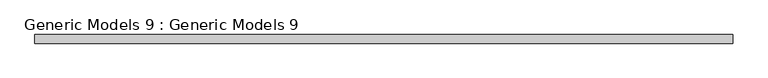
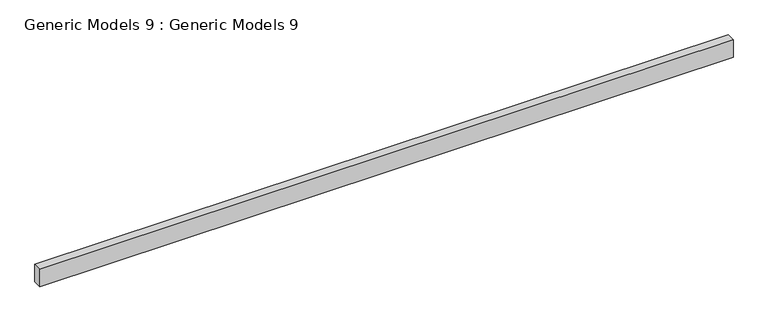
"""IFC4 building model written with IfcOpenShell, lengths in millimetres: proxy geometry, Generic Models 9 : Generic Models 9."""

from ifc_helpers import new_model, si_unit, frame, origin, place, context, project, spatial, polyline, outline, extrude, source, transform, mapped, element, save


def generic_models_9_generic_models_9_d1048e86(model_context):
    return source(origin(), model_context, "Body", "SweptSolid", [
        extrude(outline(polyline([(12604.4370151, -3682.5004242), (12604.4370151, -3949.5190062), (-8934.7629849, -3949.5190062), (-8934.7629849, -3682.5004242), (12604.4370151, -3682.5004242)])), frame((0.0, 0.0, 22668.0163948), z_axis=(0.0, 0.0, 1.0), x_axis=(1.0, 0.0, 0.0)), (0.0, 0.0, 1.0), 572.9836052),
    ])


if __name__ == "__main__":
    model = new_model("IFC4")
    model_context = context("Model", 3, world=origin())
    ifc_project = project(units=[si_unit("LENGTHUNIT", "METRE", prefix="MILLI")], contexts=[model_context])
    site = spatial("IfcSite", under=ifc_project)
    building = spatial("IfcBuilding", under=site)
    placement = place(None, origin())
    generic_models_9_generic_models_9_shape = generic_models_9_generic_models_9_d1048e86(model_context)
    element("IfcBuildingElementProxy", 1, Name="Generic Models 9 : Generic Models 9", ObjectType="Generic Models 9 : Generic Models 9", at=placement, inside=building, context=model_context, shape_type="MappedRepresentation", body=[
        mapped(generic_models_9_generic_models_9_shape, transform((0.0, 0.0, 0.0), x_axis=(1.0, 0.0, 0.0), y_axis=(0.0, 1.0, 0.0), z_axis=(0.0, 0.0, 1.0))),
    ])
    save(model, "model.ifc")
